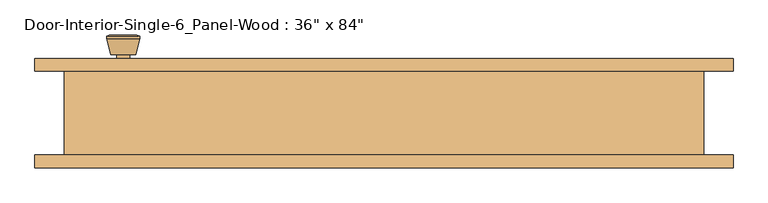
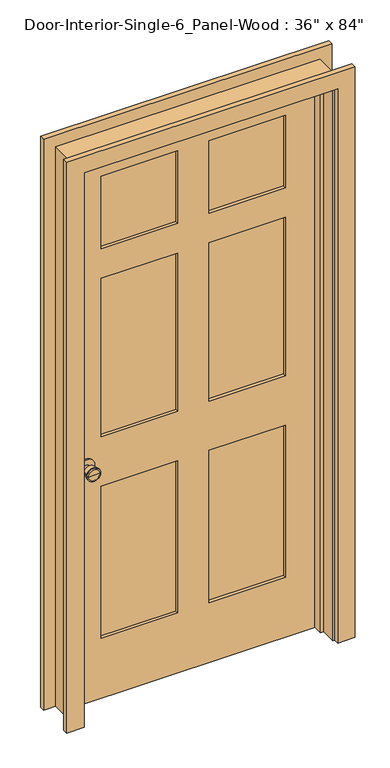
"""IFC4 building model written with IfcOpenShell, lengths in millimetres: door geometry."""

from ifc_helpers import new_model, si_unit, point, frame, frame_2d, origin, place, context, project, spatial, polyline, circle_curve, trimmed, segment, composite_curve, outline, extrude, faceted_brep, source, transform, mapped, element, save
from ifc_brep_helpers import plane_surface, cylinder_surface, revolved_surface, advanced_brep


def door_03e3dfb5(model_context):
    return source(origin(), model_context, "Body", "SolidModel", [
        advanced_brep(
        [(-393.7, 19.4, 914.4), (-383.7, 19.4, 914.4), (-403.7, 19.4, 914.4), (-373.2241324, -29.6, 914.4), (-393.7, -29.6, 914.4), (-414.1758676, -29.6, 914.4), (-368.7, -27.7721319, 914.4), (-418.7, -27.7721319, 914.4), (-368.7, -24.3084537, 914.4), (-418.7, -24.3084537, 914.4), (-375.063764, 0.4, 914.4), (-412.336236, 0.4, 914.4), (-383.7, 0.4, 914.4), (-403.7, 0.4, 914.4)],
        [
            (0, 1),
            (1, 2, circle_curve(frame((-393.7, 19.4, 914.4), z_axis=(0.0, 1.0, 0.0), x_axis=(-1.0, 0.0, 0.0)), 10.0)),
            (2, 0),
            (2, 1, circle_curve(frame((-393.7, 19.4, 914.4), z_axis=(0.0, 1.0, 0.0), x_axis=(-1.0, 0.0, 0.0)), 10.0)),
            (3, 4),
            (4, 5),
            (5, 3, circle_curve(frame((-393.7, -29.6, 914.4), z_axis=(0.0, -1.0, 0.0), x_axis=(-1.0, 0.0, 0.0)), 20.4758676)),
            (3, 5, circle_curve(frame((-393.7, -29.6, 914.4), z_axis=(0.0, -1.0, 0.0), x_axis=(-1.0, 0.0, 0.0)), 20.4758676)),
            (6, 3),
            (5, 7),
            (7, 6, circle_curve(frame((-393.7, -27.7721319, 914.4), z_axis=(0.0, -1.0, 0.0), x_axis=(-1.0, 0.0, 0.0)), 25.0)),
            (6, 7, circle_curve(frame((-393.7, -27.7721319, 914.4), z_axis=(0.0, -1.0, 0.0), x_axis=(-1.0, 0.0, 0.0)), 25.0)),
            (8, 6),
            (7, 9),
            (9, 8, circle_curve(frame((-393.7, -24.3084537, 914.4), z_axis=(0.0, -1.0, 0.0), x_axis=(-1.0, 0.0, 0.0)), 25.0)),
            (8, 9, circle_curve(frame((-393.7, -24.3084537, 914.4), z_axis=(0.0, -1.0, 0.0), x_axis=(-1.0, 0.0, 0.0)), 25.0)),
            (10, 8),
            (9, 11),
            (11, 10, circle_curve(frame((-393.7, 0.4, 914.4), z_axis=(0.0, -1.0, 0.0), x_axis=(-1.0, 0.0, 0.0)), 18.636236)),
            (10, 11, circle_curve(frame((-393.7, 0.4, 914.4), z_axis=(0.0, -1.0, 0.0), x_axis=(-1.0, 0.0, 0.0)), 18.636236)),
            (12, 10),
            (11, 13),
            (13, 12, circle_curve(frame((-393.7, 0.4, 914.4), z_axis=(0.0, -1.0, 0.0), x_axis=(-1.0, 0.0, 0.0)), 10.0)),
            (12, 13, circle_curve(frame((-393.7, 0.4, 914.4), z_axis=(0.0, -1.0, 0.0), x_axis=(-1.0, 0.0, 0.0)), 10.0)),
            (1, 12),
            (13, 2),
        ],
        [
            plane_surface(frame((-393.7, 19.4, 914.4), z_axis=(0.0, 1.0, 0.0), x_axis=(-1.0, 0.0, 0.0))),
            plane_surface(frame((-393.7, -29.6, 914.4), z_axis=(0.0, -1.0, 0.0), x_axis=(-1.0, 0.0, 0.0))),
            revolved_surface(polyline([(-414.1758676, -29.6, 914.4), (-418.7, -27.7721319, 914.4)]), (-393.7, 19.4, 914.4), (0.0, 1.0, 0.0)),
            cylinder_surface(frame((-393.7, 19.4, 914.4), z_axis=(0.0, 1.0, 0.0), x_axis=(-1.0, 0.0, 0.0)), 25.0),
            revolved_surface(polyline([(-418.7, -24.3084537, 914.4), (-412.336236, 0.4, 914.4)]), (-393.7, 19.4, 914.4), (0.0, 1.0, 0.0)),
            plane_surface(frame((-393.7, 0.4, 914.4), z_axis=(0.0, 1.0, 0.0), x_axis=(-1.0, 0.0, 0.0))),
            cylinder_surface(frame((-393.7, 19.4, 914.4), z_axis=(0.0, 1.0, 0.0), x_axis=(-1.0, 0.0, 0.0)), 10.0),
        ],
        [
            (0, [[1, 2, 3]]),
            (0, [[-3, 4, -1]]),
            (1, [[5, 6, 7]]),
            (1, [[-6, -5, 8]]),
            (2, [[9, -7, 10, 11]]),
            (2, [[-10, -8, -9, 12]]),
            (3, [[13, -11, 14, 15]]),
            (3, [[-14, -12, -13, 16]]),
            (4, [[17, -15, 18, 19]]),
            (4, [[-18, -16, -17, 20]]),
            (5, [[21, -19, 22, 23]]),
            (5, [[-22, -20, -21, 24]]),
            (6, [[25, -23, 26, -2]]),
            (6, [[-26, -24, -25, -4]]),
        ],
    ),
        extrude(outline(composite_curve([segment(trimmed(circle_curve(frame_2d((914.4, -393.7)), 30.0), [point((914.4, -423.7))], [point((914.4, -363.7))], False, "CARTESIAN"), True, "CONTINUOUS"), segment(trimmed(circle_curve(frame_2d((914.4, -393.7)), 30.0), [point((914.4, -363.7))], [point((914.4, -423.7))], False, "CARTESIAN"), True, "CONTINUOUS")], self_intersect=False)), frame((0.0, 19.4, 0.0), z_axis=(0.0, 1.0, 0.0), x_axis=(0.0, 0.0, 1.0)), (0.0, 0.0, 1.0), 6.0),
        advanced_brep(
        [(-393.7, 66.325, 914.4), (-403.7, 66.325, 914.4), (-383.7, 66.325, 914.4), (-373.2241324, 115.325, 914.4), (-414.1758676, 115.325, 914.4), (-393.7, 115.325, 914.4), (-368.7, 113.4971319, 914.4), (-418.7, 113.4971319, 914.4), (-368.7, 110.0334537, 914.4), (-418.7, 110.0334537, 914.4), (-375.063764, 85.325, 914.4), (-412.336236, 85.325, 914.4), (-383.7, 85.325, 914.4), (-403.7, 85.325, 914.4)],
        [
            (0, 1),
            (1, 2, circle_curve(frame((-393.7, 66.325, 914.4), z_axis=(0.0, -1.0, 0.0), x_axis=(-1.0, 0.0, 0.0)), 10.0)),
            (2, 0),
            (2, 1, circle_curve(frame((-393.7, 66.325, 914.4), z_axis=(0.0, -1.0, 0.0), x_axis=(-1.0, 0.0, 0.0)), 10.0)),
            (3, 4, circle_curve(frame((-393.7, 115.325, 914.4), z_axis=(0.0, 1.0, 0.0), x_axis=(-1.0, 0.0, 0.0)), 20.4758676)),
            (4, 5),
            (5, 3),
            (4, 3, circle_curve(frame((-393.7, 115.325, 914.4), z_axis=(0.0, 1.0, 0.0), x_axis=(-1.0, 0.0, 0.0)), 20.4758676)),
            (6, 7, circle_curve(frame((-393.7, 113.4971319, 914.4), z_axis=(0.0, 1.0, 0.0), x_axis=(-1.0, 0.0, 0.0)), 25.0)),
            (7, 4),
            (3, 6),
            (7, 6, circle_curve(frame((-393.7, 113.4971319, 914.4), z_axis=(0.0, 1.0, 0.0), x_axis=(-1.0, 0.0, 0.0)), 25.0)),
            (8, 9, circle_curve(frame((-393.7, 110.0334537, 914.4), z_axis=(0.0, 1.0, 0.0), x_axis=(-1.0, 0.0, 0.0)), 25.0)),
            (9, 7),
            (6, 8),
            (9, 8, circle_curve(frame((-393.7, 110.0334537, 914.4), z_axis=(0.0, 1.0, 0.0), x_axis=(-1.0, 0.0, 0.0)), 25.0)),
            (10, 11, circle_curve(frame((-393.7, 85.325, 914.4), z_axis=(0.0, 1.0, 0.0), x_axis=(-1.0, 0.0, 0.0)), 18.636236)),
            (11, 9),
            (8, 10),
            (11, 10, circle_curve(frame((-393.7, 85.325, 914.4), z_axis=(0.0, 1.0, 0.0), x_axis=(-1.0, 0.0, 0.0)), 18.636236)),
            (12, 13, circle_curve(frame((-393.7, 85.325, 914.4), z_axis=(0.0, 1.0, 0.0), x_axis=(-1.0, 0.0, 0.0)), 10.0)),
            (13, 11),
            (10, 12),
            (13, 12, circle_curve(frame((-393.7, 85.325, 914.4), z_axis=(0.0, 1.0, 0.0), x_axis=(-1.0, 0.0, 0.0)), 10.0)),
            (1, 13),
            (12, 2),
        ],
        [
            plane_surface(frame((-393.7, 66.325, 914.4), z_axis=(0.0, -1.0, 0.0), x_axis=(-1.0, 0.0, 0.0))),
            plane_surface(frame((-393.7, 115.325, 914.4), z_axis=(0.0, 1.0, 0.0), x_axis=(-1.0, 0.0, 0.0))),
            revolved_surface(polyline([(-414.1758676, 115.325, 914.4), (-418.7, 113.4971319, 914.4)]), (-393.7, 66.325, 914.4), (0.0, -1.0, 0.0)),
            cylinder_surface(frame((-393.7, 66.325, 914.4), z_axis=(0.0, -1.0, 0.0), x_axis=(-1.0, 0.0, 0.0)), 25.0),
            revolved_surface(polyline([(-418.7, 110.0334537, 914.4), (-412.336236, 85.325, 914.4)]), (-393.7, 66.325, 914.4), (0.0, -1.0, 0.0)),
            plane_surface(frame((-393.7, 85.325, 914.4), z_axis=(0.0, -1.0, 0.0), x_axis=(-1.0, 0.0, 0.0))),
            cylinder_surface(frame((-393.7, 66.325, 914.4), z_axis=(0.0, -1.0, 0.0), x_axis=(-1.0, 0.0, 0.0)), 10.0),
        ],
        [
            (0, [[1, 2, 3]]),
            (0, [[-3, 4, -1]]),
            (1, [[5, 6, 7]]),
            (1, [[8, -7, -6]]),
            (2, [[9, 10, -5, 11]]),
            (2, [[12, -11, -8, -10]]),
            (3, [[13, 14, -9, 15]]),
            (3, [[16, -15, -12, -14]]),
            (4, [[17, 18, -13, 19]]),
            (4, [[20, -19, -16, -18]]),
            (5, [[21, 22, -17, 23]]),
            (5, [[24, -23, -20, -22]]),
            (6, [[-2, 25, -21, 26]]),
            (6, [[-4, -26, -24, -25]]),
        ],
    ),
        extrude(outline(composite_curve([segment(trimmed(circle_curve(frame_2d((914.4, -393.7)), 30.0), [point((914.4, -423.7))], [point((914.4, -363.7))], False, "CARTESIAN"), True, "CONTINUOUS"), segment(trimmed(circle_curve(frame_2d((914.4, -393.7)), 30.0), [point((914.4, -363.7))], [point((914.4, -423.7))], False, "CARTESIAN"), True, "CONTINUOUS")], self_intersect=False)), frame((0.0, 60.325, 0.0), z_axis=(0.0, 1.0, 0.0), x_axis=(0.0, 0.0, 1.0)), (0.0, 0.0, 1.0), 6.0),
        faceted_brep([(482.6, 60.325, 0.0), (482.6, -66.675, 0.0), (457.2, -66.675, 0.0), (457.2, -9.525, 0.0), (444.5, -9.525, 0.0), (444.5, 25.4, 0.0), (457.2, 25.4, 0.0), (457.2, 60.325, 0.0), (482.6, 60.325, 2159.0), (482.6, -66.675, 2159.0), (-482.6, -66.675, 2159.0), (-482.6, -66.675, 0.0), (-457.2, -66.675, 0.0), (-457.2, -66.675, 2133.6), (457.2, -66.675, 2133.6), (457.2, -9.525, 2133.6), (-457.2, -9.525, 2133.6), (-457.2, -9.525, 0.0), (-444.5, -9.525, 0.0), (-444.5, -9.525, 2120.9), (444.5, -9.525, 2120.9), (444.5, 25.4, 2120.9), (-444.5, 25.4, 2120.9), (-444.5, 25.4, 0.0), (-457.2, 25.4, 0.0), (-457.2, 25.4, 2133.6), (457.2, 25.4, 2133.6), (457.2, 60.325, 2133.6), (-457.2, 60.325, 2133.6), (-457.2, 60.325, 0.0), (-482.6, 60.325, 0.0), (-482.6, 60.325, 2159.0)], [[[0, 1, 2, 3, 4, 5, 6, 7]], [[1, 0, 8, 9]], [[2, 1, 9, 10, 11, 12, 13, 14]], [[3, 2, 14, 15]], [[4, 3, 15, 16, 17, 18, 19, 20]], [[5, 4, 20, 21]], [[6, 5, 21, 22, 23, 24, 25, 26]], [[7, 6, 26, 27]], [[0, 7, 27, 28, 29, 30, 31, 8]], [[9, 8, 31, 10]], [[15, 14, 13, 16]], [[21, 20, 19, 22]], [[27, 26, 25, 28]], [[30, 29, 24, 23, 18, 17, 12, 11]], [[10, 31, 30, 11]], [[16, 13, 12, 17]], [[22, 19, 18, 23]], [[28, 25, 24, 29]]]),
        extrude(outline(polyline([(2133.6, -457.2), (0.0, -457.2), (0.0, 457.2), (2133.6, 457.2), (2133.6, -457.2)]), holes=[polyline([(2014.5375, 57.15), (2014.5375, 336.55), (1735.1375, 336.55), (1735.1375, 57.15), (2014.5375, 57.15)]), polyline([(1620.8375, 336.55), (1009.65, 336.55), (1009.65, 57.15), (1620.8375, 57.15), (1620.8375, 336.55)]), polyline([(1009.65, -57.15), (1009.65, -336.55), (1620.8375, -336.55), (1620.8375, -57.15), (1009.65, -57.15)]), polyline([(1735.1375, -336.55), (2014.5375, -336.55), (2014.5375, -57.15), (1735.1375, -57.15), (1735.1375, -336.55)]), polyline([(819.15, 57.15), (819.15, 336.55), (231.775, 336.55), (231.775, 57.15), (819.15, 57.15)]), polyline([(231.775, -57.15), (231.775, -336.55), (819.15, -336.55), (819.15, -57.15), (231.775, -57.15)])]), frame((0.0, 25.4, 0.0), z_axis=(0.0, 1.0, 0.0), x_axis=(0.0, 0.0, 1.0)), (0.0, 0.0, 1.0), 34.925),
        extrude(outline(polyline([(336.55, 37.0416667), (57.15, 37.0416667), (57.15, 48.6833333), (336.55, 48.6833333), (336.55, 37.0416667)])), frame((0.0, 0.0, 1735.1375), z_axis=(0.0, 0.0, 1.0), x_axis=(1.0, 0.0, 0.0)), (0.0, 0.0, 1.0), 279.4),
        extrude(outline(polyline([(336.55, 37.0416667), (57.15, 37.0416667), (57.15, 48.6833333), (336.55, 48.6833333), (336.55, 37.0416667)])), frame((0.0, 0.0, 1009.65), z_axis=(0.0, 0.0, 1.0), x_axis=(1.0, 0.0, 0.0)), (0.0, 0.0, 1.0), 611.1875),
        extrude(outline(polyline([(-57.15, 37.0416667), (-336.55, 37.0416667), (-336.55, 48.6833333), (-57.15, 48.6833333), (-57.15, 37.0416667)])), frame((0.0, 0.0, 1009.65), z_axis=(0.0, 0.0, 1.0), x_axis=(1.0, 0.0, 0.0)), (0.0, 0.0, 1.0), 611.1875),
        extrude(outline(polyline([(-57.15, 37.0416667), (-336.55, 37.0416667), (-336.55, 48.6833333), (-57.15, 48.6833333), (-57.15, 37.0416667)])), frame((0.0, 0.0, 1735.1375), z_axis=(0.0, 0.0, 1.0), x_axis=(1.0, 0.0, 0.0)), (0.0, 0.0, 1.0), 279.4),
        extrude(outline(polyline([(336.55, 37.0416667), (57.15, 37.0416667), (57.15, 48.6833333), (336.55, 48.6833333), (336.55, 37.0416667)])), frame((0.0, 0.0, 231.775), z_axis=(0.0, 0.0, 1.0), x_axis=(1.0, 0.0, 0.0)), (0.0, 0.0, 1.0), 587.375),
        extrude(outline(polyline([(-57.15, 37.0416667), (-336.55, 37.0416667), (-336.55, 48.6833333), (-57.15, 48.6833333), (-57.15, 37.0416667)])), frame((0.0, 0.0, 231.775), z_axis=(0.0, 0.0, 1.0), x_axis=(1.0, 0.0, 0.0)), (0.0, 0.0, 1.0), 587.375),
        extrude(outline(polyline([(0.0, 463.55), (0.0, 527.05), (2203.45, 527.05), (2203.45, -527.05), (0.0, -527.05), (0.0, -463.55), (2139.95, -463.55), (2139.95, 463.55), (0.0, 463.55)])), frame((0.0, 60.325, 0.0), z_axis=(0.0, 1.0, 0.0), x_axis=(0.0, 0.0, 1.0)), (0.0, 0.0, 1.0), 19.05),
        extrude(outline(polyline([(0.0, 463.55), (0.0, 527.05), (2203.45, 527.05), (2203.45, -527.05), (0.0, -527.05), (0.0, -463.55), (2139.95, -463.55), (2139.95, 463.55), (0.0, 463.55)])), frame((0.0, -85.725, 0.0), z_axis=(0.0, 1.0, 0.0), x_axis=(0.0, 0.0, 1.0)), (0.0, 0.0, 1.0), 19.05),
    ])


if __name__ == "__main__":
    model = new_model("IFC4")
    model_context = context("Model", 3, world=origin())
    ifc_project = project(units=[si_unit("LENGTHUNIT", "METRE", prefix="MILLI")], contexts=[model_context])
    site = spatial("IfcSite", under=ifc_project)
    building = spatial("IfcBuilding", under=site)
    placement = place(None, origin())
    door_shape = door_03e3dfb5(model_context)
    element("IfcDoor", 1, ObjectType="Door-Interior-Single-6_Panel-Wood : 36\" x 84\"", at=placement, inside=building, context=model_context, shape_type="MappedRepresentation", body=[
        mapped(door_shape, transform((0.0, 0.0, 0.0), x_axis=(1.0, 0.0, 0.0), y_axis=(0.0, 1.0, 0.0), z_axis=(0.0, 0.0, 1.0))),
    ])
    save(model, "model.ifc")

# Revit data of these elements
# Type "Door-Interior-Single-6_Panel-Wood : 36\" x 84\""
#   Type Mark = "8"
#   Assembly Code = "C1020300"
#   Analytic Construction = "Wooden"
#   Top Rail = 0' - 4 11/16"
#   Top Panel = 0' - 11"
#   Thickness = 0' - 1 3/8"
#   Thermal Resistance (R) = 2.5876 (h·ft²·°F)/BTU
#   Swing Angle [instance default] = 90.00°
#   Stiles = 0' - 4 3/4"
#   Rough Width = 3' - 2"
#   Rough Height = 7' - 1"
#   Mullion = 0' - 4 1/2"
#   Lock Rail = 0' - 7 1/2"
#   Intermediate Rail = 0' - 4 1/2"
#   Height = 7' - 0"
#   Width = 3' - 0"
#   Heat Transfer Coefficient (U) = 0.3865 BTU/(h·ft²·°F)
#   Bottom Rail = 0' - 9 1/8"
#   Trim Material = Cherry
#   Panel Material = Cherry
#   Frame Material = Cherry
#   Door Handle Material = Aluminum
#   Visual Light Transmittance = 0
#   Solar Heat Gain Coefficient = 0
#   Wall Closure = (empty or 0)
#   Function = (empty or 0)
# Element 1 (IfcDoor, "Door-Interior-Single-6_Panel-Wood : 36\" x 84\"")
#   Materials on its faces: "Cherry", "Aluminum"
# Materials
#   "Cherry": class "Wood", colour RGB 226 177 128, transparency 0, Description = "Prunus Serotina", Cost = 0
#   "Aluminum": class "Metal", colour RGB 247 247 247, transparency 0, Description = "Aluminum 6061", Cost = 0
